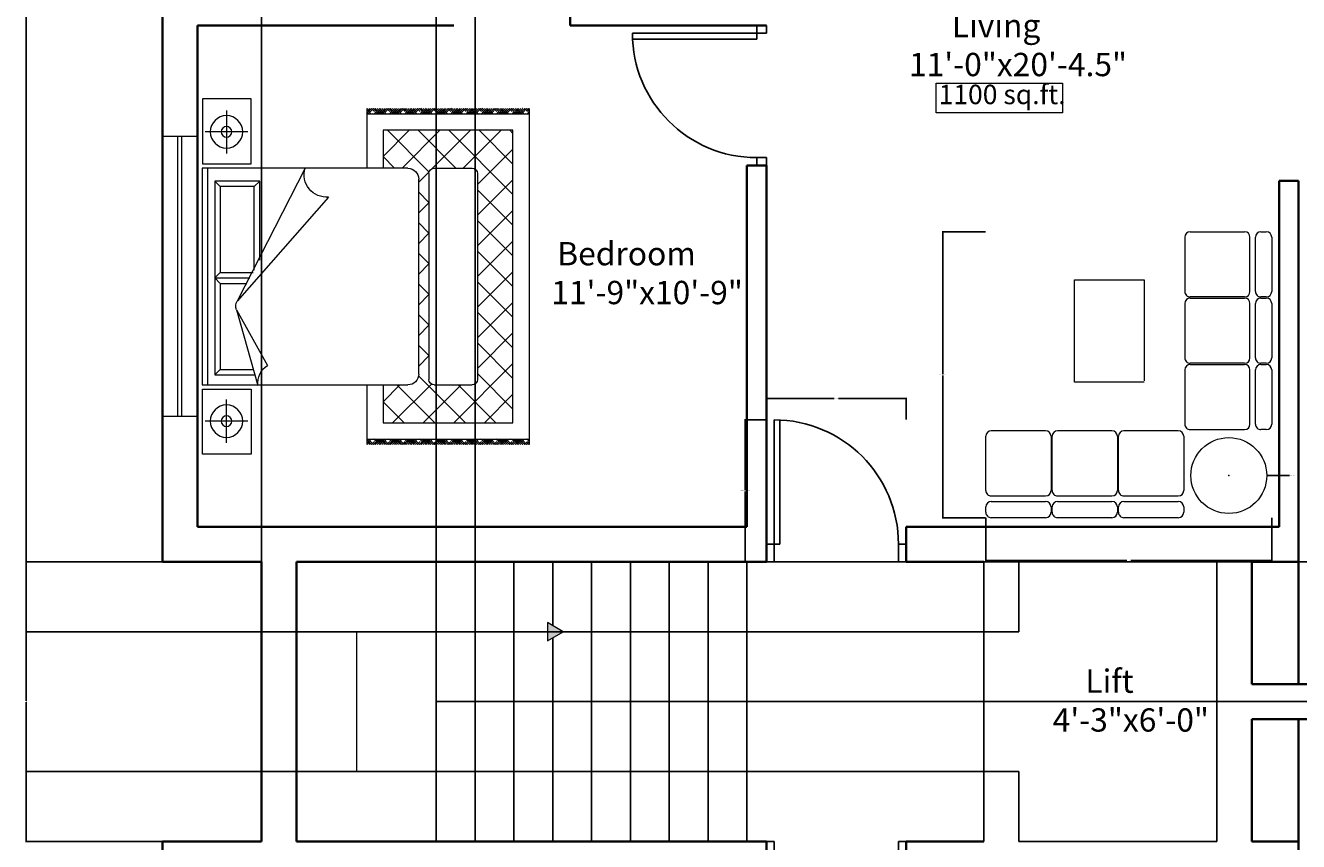
# Model space of a CAD drawing. Units: inches. Extents: x 3198 to 3702, y 1509 to 2253.
# Tile 4 of 6: x 3198 to 3526, y 1845 to 2055. Entities that reach past the tile are written whole.
import ezdxf

# ---------------------------------------------------------------- set-up
doc = ezdxf.new("R2010")
doc.units = ezdxf.units.IN
for name, color, linetype, lineweight in [('A-ANNO-DIMS', 2, 'Continuous', 18), ('A-ANNO-SYMB', 7, 'Continuous', 18), ('A-AREA-IDEN', 7, 'Continuous', 18), ('A-DOOR', 3, 'Continuous', 25), ('A-FLOR-EVTR', 7, 'Continuous', 25), ('A-FLOR-STRS', 7, 'Continuous', 25), ('A-FURN', 8, 'Continuous', 13), ('A-GLAZ', 4, 'Continuous', 18), ('A-WALL', 7, 'Continuous', 35)]:
    doc.layers.add(name, color=color, linetype=linetype, lineweight=lineweight)
doc.styles.get("Standard").update_dxf_attribs({"font": 'arial.ttf'})
doc.dimstyles.get("Standard").update_dxf_attribs({"dimtxt": 0.18, "dimasz": 0.18, "dimexe": 0.18, "dimexo": 0.0625, "dimgap": 0.09, "dimtad": 0, "dimtih": 1, "dimtoh": 1, "dimdec": 4, "dimzin": 0, "dimdsep": 46, "dimtxsty": 'Standard', "dimcen": 0.09, "dimadec": 0, "dimazin": 0, "dimtfac": 1, "dimtdec": 4, "dimtofl": 0, "dimtmove": 0, "dimatfit": 3, "dimfxl": 1, "dimtolj": 1, "dimtzin": 0, "dimarcsym": 0})

# ---------------------------------------------------------------- blocks, each defined once
blk = doc.blocks.new('A$C753D6792')
at = {"linetype": 'ByBlock'}
for p, q in [((0, 2530), (0, 2580)), ((50, 2630), (550, 2630)), ((600, 2580), (600, 2530)), ((610, 2530), (610, 2580)), ((660, 2630), (1160, 2630)), ((1210, 2580), (1210, 2530)), ((1220, 2530), (1220, 2580)), ((1270, 2630), (1770, 2630)), ((1820, 2580), (1820, 2530)), ((550, 2480), (50, 2480)), ((1160, 2480), (660, 2480)), ((1770, 2480), (1270, 2480)), ((0, 1880), (0, 2380)), ((550, 2430), (50, 2430)), ((600, 2380), (600, 1880)), ((610, 1880), (610, 2380)), ((1160, 2430), (660, 2430)), ((1210, 2380), (1210, 1880)), ((1220, 1880), (1220, 2380)), ((1770, 2430), (1270, 2430)), ((1820, 1880), (1820, 2380)), ((50, 1830), (427, 1830)), ((387, 1830), (550, 1830)), ((660, 1830), (1037, 1830)), ((997, 1830), (1160, 1830)), ((1270, 1830), (1647, 1830)), ((1607, 1830), (1770, 1830)), ((1830, 1770), (1830, 1393)), ((1880, 1820), (2380, 1820)), ((2430, 1270), (2430, 1770)), ((2480, 1270), (2480, 1770)), ((2530, 1820), (2580, 1820)), ((2630, 1770), (2630, 1270)), ((442, 815), (442, 1455)), ((442, 1455), (1372, 1455)), ((1382, 1455), (1382, 815)), ((1830, 1433), (1830, 1270)), ((2380, 1220), (1880, 1220)), ((1880, 1210), (2380, 1210)), ((2580, 1220), (2530, 1220)), ((2530, 1210), (2580, 1210)), ((1830, 1160), (1830, 783)), ((2430, 660), (2430, 1160)), ((2480, 660), (2480, 1160)), ((2630, 1160), (2630, 660)), ((1830, 823), (1830, 660)), ((1382, 815), (442, 815)), ((2380, 610), (1880, 610)), ((1880, 600), (2380, 600)), ((2580, 610), (2530, 610)), ((2530, 600), (2580, 600)), ((1830, 550), (1830, 173)), ((2430, 50), (2430, 550)), ((2480, 50), (2480, 550)), ((2630, 550), (2630, 50)), ((1830, 213), (1830, 50)), ((2380, 0), (1880, 0)), ((2580, 0), (2530, 0))]:
    blk.add_line(p, q, dxfattribs=at)
blk.add_circle((2242, 2235), 349, dxfattribs=at)
for centre, start, end in [((50, 2580), 90, 180), ((550, 2580), 0, 90), ((550, 2580), 0, 90), ((660, 2580), 90, 180), ((1160, 2580), 0, 90), ((1160, 2580), 0, 90), ((1270, 2580), 90, 180), ((1770, 2580), 0, 90), ((1770, 2580), 0, 90), ((50, 2530), 180, 270), ((550, 2530), 270, 0), ((550, 2530), 270, 0), ((660, 2530), 180, 270), ((1160, 2530), 270, 0), ((1160, 2530), 270, 0), ((1270, 2530), 180, 270), ((1770, 2530), 270, 0), ((1770, 2530), 270, 0), ((50, 2380), 90, 180), ((550, 2380), 0, 90), ((550, 2380), 0, 90), ((660, 2380), 90, 180), ((1160, 2380), 0, 90), ((1160, 2380), 0, 90), ((1270, 2380), 90, 180), ((1770, 2380), 0, 90), ((1770, 2380), 0, 90), ((50, 1880), 180, 270), ((550, 1880), 270, 0), ((660, 1880), 180, 270), ((1160, 1880), 270, 0), ((1270, 1880), 180, 270), ((1770, 1880), 270, 0), ((1880, 1770), 90, 180), ((2380, 1770), 0, 90), ((2530, 1770), 90, 180), ((2580, 1770), 0, 90), ((1880, 1270), 180, 270), ((1880, 1160), 90, 180), ((2380, 1270), 270, 0), ((2380, 1270), 270, 0), ((2380, 1160), 0, 90), ((2530, 1270), 180, 270), ((2530, 1270), 180, 270), ((2530, 1160), 90, 180), ((2580, 1270), 270, 0), ((2580, 1270), 270, 0), ((2580, 1160), 0, 90), ((1880, 660), 180, 270), ((1880, 550), 90, 180), ((2380, 660), 270, 0), ((2380, 660), 270, 0), ((2380, 550), 0, 90), ((2530, 660), 180, 270), ((2530, 660), 180, 270), ((2530, 550), 90, 180), ((2580, 660), 270, 0), ((2580, 660), 270, 0), ((2580, 550), 0, 90), ((1880, 50), 180, 270), ((2380, 50), 270, 0), ((2380, 50), 270, 0), ((2530, 50), 180, 270), ((2530, 50), 180, 270), ((2580, 50), 270, 0), ((2580, 50), 270, 0)]:
    blk.add_arc(centre, 50, start, end, dxfattribs=at)
blk = doc.blocks.new('A$C4CB008C5')
for p, q in [((0, 3.019), (0.6, 3.019)), ((0, 2.569), (0, 3.019)), ((0.304, 2.6), (0.304, 2.992)), ((0.6, 3.019), (0.6, 2.569)), ((0.64, 1.121), (0.64, 3.021)), ((0.64, 3.021), (2.64, 3.021)), ((0.64, 2.971), (2.64, 2.971)), ((2.64, 3.021), (2.64, 1.121)), ((3.279, 3.019), (2.679, 3.019)), ((2.679, 3.019), (2.679, 2.569)), ((2.975, 2.6), (2.975, 2.992)), ((3.279, 2.569), (3.279, 3.019)), ((0.759, 2.905), (2.547, 2.905)), ((0.759, 2.489), (0.759, 2.905)), ((0.759, 2.905), (0.809, 2.855)), ((0.809, 2.855), (1.603, 2.855)), ((0.809, 2.539), (0.809, 2.855)), ((1.603, 2.855), (1.653, 2.905)), ((1.603, 2.855), (1.603, 2.551)), ((1.653, 2.905), (1.653, 2.579)), ((1.653, 2.905), (1.703, 2.855)), ((1.703, 2.855), (1.703, 2.607)), ((1.703, 2.855), (2.497, 2.855)), ((2.497, 2.855), (2.547, 2.905)), ((2.497, 2.855), (2.497, 2.556)), ((2.547, 2.905), (2.547, 2.54)), ((0.106, 2.796), (0.503, 2.796)), ((1.946, 2.705), (2.646, 2.507)), ((1.946, 2.705), (2.46, 2.418)), ((3.174, 2.796), (2.776, 2.796)), ((0.64, 2.071), (1.866, 2.698)), ((0.906, 1.854), (1.866, 2.698)), ((0.6, 2.569), (0, 2.569)), ((0.809, 2.539), (0.759, 2.489)), ((1.49, 2.489), (0.759, 2.489)), ((1.58, 2.539), (0.809, 2.539)), ((2.679, 2.569), (3.279, 2.569)), ((0.907, 1.867), (0.919, 1.867)), ((0.09, 1.5), (0.64, 1.5)), ((0.09, 1.491), (0.099, 1.5)), ((0.09, 1.473), (0.116, 1.5)), ((0.09, 1.456), (0.134, 1.5)), ((0.09, 1.474), (0.09, 1.475)), ((0.09, 1.438), (0.126, 1.474)), ((0.117, 1.43), (0.09, 1.457)), ((0.14, 1.389), (0.09, 1.439)), ((0.09, 1.42), (0.099, 1.43)), ((0.14, 1.372), (0.09, 1.422)), ((0.09, 1.368), (0.14, 1.417)), ((0.14, 1.46), (0.108, 1.492)), ((0.117, 1.412), (0.14, 1.435)), ((0.14, 1.478), (0.118, 1.5)), ((0.14, 1.496), (0.135, 1.5)), ((0.14, 1.442), (0.135, 1.448)), ((0.14, 0), (0.14, 1.5)), ((2.64, 1.5), (3.19, 1.5)), ((3.14, 1.496), (3.144, 1.5)), ((3.14, 1.478), (3.162, 1.5)), ((3.14, 1.5), (3.14, 0)), ((3.14, 1.46), (3.171, 1.492)), ((3.14, 1.442), (3.145, 1.448)), ((3.14, 1.389), (3.19, 1.439)), ((3.162, 1.412), (3.14, 1.435)), ((3.14, 1.372), (3.19, 1.422)), ((3.189, 1.368), (3.14, 1.417)), ((3.19, 1.456), (3.145, 1.5)), ((3.19, 1.438), (3.154, 1.474)), ((3.162, 1.43), (3.19, 1.457)), ((3.19, 1.473), (3.163, 1.5)), ((3.19, 1.42), (3.18, 1.43)), ((3.19, 1.491), (3.181, 1.5)), ((3.189, 1.474), (3.19, 1.475)), ((0.14, 1.354), (0.09, 1.404)), ((0.09, 1.35), (0.14, 1.4)), ((0.14, 1.336), (0.09, 1.386)), ((0.09, 1.332), (0.14, 1.382)), ((0.09, 1.314), (0.14, 1.364)), ((0.09, 1.297), (0.126, 1.333)), ((0.09, 1.333), (0.09, 1.333)), ((0.117, 1.288), (0.09, 1.316)), ((0.14, 1.248), (0.09, 1.298)), ((0.14, 1.319), (0.108, 1.35)), ((0.117, 1.271), (0.14, 1.294)), ((0.14, 1.301), (0.135, 1.306)), ((0.29, 1.108), (0.532, 1.35)), ((0.29, 0.15), (0.29, 1.35)), ((0.29, 1.35), (0.64, 1.35)), ((0.674, 0.926), (0.29, 1.31)), ((0.64, 1.243), (0.533, 1.35)), ((2.64, 1.195), (2.795, 1.35)), ((2.64, 1.35), (2.99, 1.35)), ((2.99, 1.156), (2.795, 1.35)), ((2.99, 1.35), (2.99, 0.15)), ((3.14, 1.354), (3.19, 1.404)), ((3.19, 1.35), (3.14, 1.4)), ((3.14, 1.336), (3.19, 1.386)), ((3.19, 1.332), (3.14, 1.382)), ((3.19, 1.314), (3.14, 1.364)), ((3.14, 1.319), (3.171, 1.35)), ((3.14, 1.301), (3.145, 1.306)), ((3.14, 1.248), (3.19, 1.298)), ((3.162, 1.271), (3.14, 1.294)), ((3.19, 1.297), (3.154, 1.333)), ((3.162, 1.288), (3.19, 1.316)), ((3.189, 1.333), (3.19, 1.333)), ((0.09, 1.279), (0.099, 1.288)), ((0.14, 1.23), (0.09, 1.28)), ((0.09, 1.227), (0.14, 1.276)), ((0.14, 1.213), (0.09, 1.263)), ((0.09, 1.208), (0.14, 1.258)), ((0.14, 1.195), (0.09, 1.245)), ((0.09, 1.19), (0.14, 1.24)), ((0.09, 1.173), (0.14, 1.223)), ((0.09, 1.191), (0.09, 1.192)), ((0.09, 1.155), (0.126, 1.191)), ((0.14, 1.177), (0.108, 1.209)), ((2.632, 0.904), (2.99, 1.262)), ((2.99, 0.873), (2.64, 1.223)), ((3.14, 1.23), (3.19, 1.28)), ((3.189, 1.227), (3.14, 1.276)), ((3.14, 1.213), (3.19, 1.263)), ((3.19, 1.208), (3.14, 1.258)), ((3.14, 1.195), (3.19, 1.245)), ((3.19, 1.19), (3.14, 1.24)), ((3.19, 1.173), (3.14, 1.223)), ((3.14, 1.177), (3.171, 1.209)), ((3.19, 1.155), (3.154, 1.191)), ((3.19, 1.279), (3.18, 1.288)), ((3.189, 1.191), (3.19, 1.192)), ((0.117, 1.147), (0.09, 1.174)), ((0.14, 1.107), (0.09, 1.157)), ((0.09, 1.137), (0.099, 1.147)), ((0.14, 1.089), (0.09, 1.139)), ((0.09, 1.085), (0.14, 1.134)), ((0.14, 1.071), (0.09, 1.121)), ((0.09, 1.067), (0.14, 1.117)), ((0.14, 1.054), (0.09, 1.104)), ((0.09, 1.049), (0.14, 1.099)), ((0.09, 1.031), (0.14, 1.081)), ((0.14, 1.036), (0.108, 1.067)), ((0.117, 1.129), (0.14, 1.152)), ((0.14, 1.16), (0.135, 1.165)), ((0.29, 0.825), (0.64, 1.175)), ((3.14, 1.16), (3.145, 1.165)), ((3.14, 1.107), (3.19, 1.157)), ((3.162, 1.129), (3.14, 1.152)), ((3.14, 1.089), (3.19, 1.139)), ((3.189, 1.085), (3.14, 1.134)), ((3.14, 1.071), (3.19, 1.121)), ((3.19, 1.067), (3.14, 1.117)), ((3.14, 1.054), (3.19, 1.104)), ((3.19, 1.049), (3.14, 1.099)), ((3.19, 1.031), (3.14, 1.081)), ((3.14, 1.036), (3.171, 1.067)), ((3.162, 1.147), (3.19, 1.174)), ((3.19, 1.137), (3.18, 1.147)), ((0.09, 1.05), (0.09, 1.051)), ((0.09, 1.014), (0.126, 1.05)), ((0.117, 1.006), (0.09, 1.033)), ((0.14, 0.965), (0.09, 1.015)), ((0.09, 0.996), (0.099, 1.006)), ((0.14, 0.948), (0.09, 0.998)), ((0.09, 0.944), (0.14, 0.993)), ((0.14, 0.93), (0.09, 0.98)), ((0.09, 0.925), (0.14, 0.975)), ((0.14, 0.912), (0.09, 0.962)), ((0.09, 0.908), (0.14, 0.958)), ((0.117, 0.988), (0.14, 1.011)), ((0.14, 1.018), (0.135, 1.023)), ((0.64, 0.677), (0.29, 1.027)), ((0.673, 0.925), (0.769, 1.021)), ((2.54, 1.021), (0.74, 1.021)), ((0.955, 0.928), (0.861, 1.021)), ((0.959, 0.928), (1.052, 1.021)), ((1.238, 0.928), (1.144, 1.021)), ((1.241, 0.928), (1.335, 1.021)), ((1.52, 0.928), (1.427, 1.021)), ((1.524, 0.928), (1.618, 1.021)), ((1.803, 0.928), (1.71, 1.021)), ((1.807, 0.928), (1.9, 1.021)), ((2.086, 0.928), (1.993, 1.021)), ((2.09, 0.928), (2.183, 1.021)), ((2.369, 0.928), (2.276, 1.021)), ((2.373, 0.928), (2.466, 1.021)), ((2.99, 0.59), (2.557, 1.023)), ((2.64, 0.629), (2.99, 0.979)), ((3.14, 1.018), (3.145, 1.023)), ((3.14, 0.965), (3.19, 1.015)), ((3.162, 0.988), (3.14, 1.011)), ((3.14, 0.948), (3.19, 0.998)), ((3.189, 0.944), (3.14, 0.993)), ((3.14, 0.93), (3.19, 0.98)), ((3.19, 0.925), (3.14, 0.975)), ((3.14, 0.912), (3.19, 0.962)), ((3.19, 0.908), (3.14, 0.958)), ((3.19, 1.014), (3.154, 1.05)), ((3.162, 1.006), (3.19, 1.033)), ((3.19, 0.996), (3.18, 1.006)), ((3.189, 1.05), (3.19, 1.051)), ((0.09, 0.89), (0.14, 0.94)), ((0.09, 0.908), (0.09, 0.909)), ((0.09, 0.872), (0.126, 0.908)), ((0.117, 0.864), (0.09, 0.891)), ((0.14, 0.824), (0.09, 0.874)), ((0.09, 0.855), (0.099, 0.864)), ((0.14, 0.806), (0.09, 0.856)), ((0.09, 0.802), (0.14, 0.852)), ((0.14, 0.788), (0.09, 0.838)), ((0.09, 0.784), (0.14, 0.834)), ((0.14, 0.894), (0.108, 0.926)), ((0.117, 0.847), (0.14, 0.869)), ((0.14, 0.877), (0.135, 0.882)), ((0.29, 0.542), (0.643, 0.895)), ((0.64, 0.878), (0.64, 0.528)), ((0.69, 0.928), (2.59, 0.928)), ((2.64, 0.878), (2.64, 0.528)), ((3.19, 0.89), (3.14, 0.94)), ((3.14, 0.894), (3.171, 0.926)), ((3.14, 0.877), (3.145, 0.882)), ((3.14, 0.824), (3.19, 0.874)), ((3.162, 0.847), (3.14, 0.869)), ((3.14, 0.806), (3.19, 0.856)), ((3.189, 0.802), (3.14, 0.852)), ((3.14, 0.788), (3.19, 0.838)), ((3.19, 0.784), (3.14, 0.834)), ((3.19, 0.872), (3.154, 0.908)), ((3.162, 0.864), (3.19, 0.891)), ((3.19, 0.855), (3.18, 0.864)), ((3.189, 0.908), (3.19, 0.909)), ((0.14, 0.771), (0.09, 0.821)), ((0.09, 0.766), (0.14, 0.816)), ((0.09, 0.749), (0.14, 0.799)), ((0.09, 0.767), (0.09, 0.768)), ((0.09, 0.731), (0.126, 0.767)), ((0.117, 0.723), (0.09, 0.75)), ((0.14, 0.682), (0.09, 0.732)), ((0.09, 0.713), (0.099, 0.723)), ((0.14, 0.665), (0.09, 0.715)), ((0.09, 0.661), (0.14, 0.71)), ((0.14, 0.753), (0.108, 0.785)), ((0.117, 0.705), (0.14, 0.728)), ((0.14, 0.735), (0.135, 0.74)), ((0.884, 0.15), (0.29, 0.744)), ((3.14, 0.771), (3.19, 0.821)), ((3.19, 0.766), (3.14, 0.816)), ((3.19, 0.749), (3.14, 0.799)), ((3.14, 0.753), (3.171, 0.785)), ((3.14, 0.735), (3.145, 0.74)), ((3.14, 0.682), (3.19, 0.732)), ((3.162, 0.705), (3.14, 0.728)), ((3.14, 0.665), (3.19, 0.715)), ((3.189, 0.661), (3.14, 0.71)), ((3.19, 0.731), (3.154, 0.767)), ((3.162, 0.723), (3.19, 0.75)), ((3.19, 0.713), (3.18, 0.723)), ((3.189, 0.767), (3.19, 0.768)), ((0.14, 0.647), (0.09, 0.697)), ((0.09, 0.642), (0.14, 0.692)), ((0.14, 0.629), (0.09, 0.679)), ((0.09, 0.625), (0.14, 0.675)), ((0.09, 0.607), (0.14, 0.657)), ((0.09, 0.589), (0.126, 0.626)), ((0.09, 0.626), (0.09, 0.626)), ((0.117, 0.581), (0.09, 0.609)), ((0.14, 0.541), (0.09, 0.591)), ((0.14, 0.612), (0.108, 0.643)), ((0.14, 0.594), (0.135, 0.599)), ((0.29, 0.259), (0.64, 0.609)), ((2.443, 0.15), (2.99, 0.696)), ((2.99, 0.307), (2.64, 0.657)), ((3.14, 0.647), (3.19, 0.697)), ((3.19, 0.642), (3.14, 0.692)), ((3.14, 0.629), (3.19, 0.679)), ((3.19, 0.625), (3.14, 0.675)), ((3.19, 0.607), (3.14, 0.657)), ((3.14, 0.612), (3.171, 0.643)), ((3.14, 0.594), (3.145, 0.599)), ((3.14, 0.541), (3.19, 0.591)), ((3.19, 0.589), (3.154, 0.626)), ((3.162, 0.581), (3.19, 0.609)), ((3.189, 0.626), (3.19, 0.626)), ((0.09, 0.572), (0.099, 0.581)), ((0.14, 0.523), (0.09, 0.573)), ((0.09, 0.519), (0.14, 0.569)), ((0.14, 0.506), (0.09, 0.556)), ((0.09, 0.501), (0.14, 0.551)), ((0.14, 0.488), (0.09, 0.538)), ((0.09, 0.483), (0.14, 0.533)), ((0.09, 0.466), (0.14, 0.516)), ((0.09, 0.484), (0.09, 0.485)), ((0.09, 0.448), (0.126, 0.484)), ((0.14, 0.47), (0.108, 0.502)), ((0.117, 0.564), (0.14, 0.586)), ((0.463, 0.15), (0.791, 0.478)), ((0.69, 0.478), (2.59, 0.478)), ((0.746, 0.15), (1.074, 0.478)), ((1.167, 0.15), (0.839, 0.478)), ((1.029, 0.15), (1.357, 0.478)), ((1.45, 0.15), (1.122, 0.478)), ((1.312, 0.15), (1.64, 0.478)), ((1.733, 0.15), (1.405, 0.478)), ((1.595, 0.15), (1.923, 0.478)), ((2.016, 0.15), (1.688, 0.478)), ((1.878, 0.15), (2.206, 0.478)), ((2.298, 0.15), (1.97, 0.478)), ((2.16, 0.15), (2.488, 0.478)), ((2.581, 0.15), (2.253, 0.478)), ((2.864, 0.15), (2.536, 0.478)), ((3.162, 0.564), (3.14, 0.586)), ((3.14, 0.523), (3.19, 0.573)), ((3.189, 0.519), (3.14, 0.569)), ((3.14, 0.506), (3.19, 0.556)), ((3.19, 0.501), (3.14, 0.551)), ((3.14, 0.488), (3.19, 0.538)), ((3.19, 0.483), (3.14, 0.533)), ((3.19, 0.466), (3.14, 0.516)), ((3.14, 0.47), (3.171, 0.502)), ((3.19, 0.448), (3.154, 0.484)), ((3.19, 0.572), (3.18, 0.581)), ((3.189, 0.484), (3.19, 0.485)), ((0.117, 0.44), (0.09, 0.467)), ((0.14, 0.399), (0.09, 0.449)), ((0.09, 0.43), (0.099, 0.44)), ((0.14, 0.382), (0.09, 0.432)), ((0.09, 0.378), (0.14, 0.427)), ((0.14, 0.364), (0.09, 0.414)), ((0.09, 0.36), (0.14, 0.41)), ((0.14, 0.346), (0.09, 0.396)), ((0.09, 0.342), (0.14, 0.392)), ((0.09, 0.324), (0.14, 0.374)), ((0.14, 0.329), (0.108, 0.36)), ((0.117, 0.422), (0.14, 0.445)), ((0.14, 0.453), (0.135, 0.458)), ((0.601, 0.15), (0.29, 0.462)), ((2.726, 0.15), (2.99, 0.414)), ((3.14, 0.453), (3.145, 0.458)), ((3.14, 0.399), (3.19, 0.449)), ((3.162, 0.422), (3.14, 0.445)), ((3.14, 0.382), (3.19, 0.432)), ((3.189, 0.378), (3.14, 0.427)), ((3.14, 0.364), (3.19, 0.414)), ((3.19, 0.36), (3.14, 0.41)), ((3.14, 0.346), (3.19, 0.396)), ((3.19, 0.342), (3.14, 0.392)), ((3.19, 0.324), (3.14, 0.374)), ((3.14, 0.329), (3.171, 0.36)), ((3.162, 0.44), (3.19, 0.467)), ((3.19, 0.43), (3.18, 0.44)), ((0.09, 0.307), (0.126, 0.343)), ((0.09, 0.343), (0.09, 0.343)), ((0.117, 0.299), (0.09, 0.326)), ((0.14, 0.258), (0.09, 0.308)), ((0.09, 0.289), (0.099, 0.299)), ((0.14, 0.24), (0.09, 0.29)), ((0.09, 0.237), (0.14, 0.286)), ((0.14, 0.223), (0.09, 0.273)), ((0.09, 0.218), (0.14, 0.268)), ((0.14, 0.205), (0.09, 0.255)), ((0.09, 0.201), (0.14, 0.251)), ((0.117, 0.281), (0.14, 0.304)), ((0.14, 0.311), (0.135, 0.316)), ((3.14, 0.311), (3.145, 0.316)), ((3.14, 0.258), (3.19, 0.308)), ((3.162, 0.281), (3.14, 0.304)), ((3.14, 0.24), (3.19, 0.29)), ((3.189, 0.237), (3.14, 0.286)), ((3.14, 0.223), (3.19, 0.273)), ((3.19, 0.218), (3.14, 0.268)), ((3.14, 0.205), (3.19, 0.255)), ((3.19, 0.201), (3.14, 0.251)), ((3.19, 0.307), (3.154, 0.343)), ((3.162, 0.299), (3.19, 0.326)), ((3.19, 0.289), (3.18, 0.299)), ((3.189, 0.343), (3.19, 0.343)), ((0.09, 0.183), (0.14, 0.233)), ((0.09, 0.201), (0.09, 0.202)), ((0.09, 0.165), (0.126, 0.201)), ((0.117, 0.157), (0.09, 0.184)), ((0.14, 0.117), (0.09, 0.167)), ((0.09, 0.148), (0.099, 0.157)), ((0.14, 0.099), (0.09, 0.149)), ((0.09, 0.095), (0.14, 0.144)), ((0.14, 0.081), (0.09, 0.131)), ((0.09, 0.077), (0.14, 0.127)), ((0.14, 0.187), (0.108, 0.219)), ((0.117, 0.139), (0.14, 0.162)), ((0.14, 0.17), (0.135, 0.175)), ((0.318, 0.15), (0.29, 0.179)), ((2.99, 0.15), (0.29, 0.15)), ((3.19, 0.183), (3.14, 0.233)), ((3.14, 0.187), (3.171, 0.219)), ((3.14, 0.17), (3.145, 0.175)), ((3.14, 0.117), (3.19, 0.167)), ((3.162, 0.139), (3.14, 0.162)), ((3.14, 0.099), (3.19, 0.149)), ((3.189, 0.095), (3.14, 0.144)), ((3.14, 0.081), (3.19, 0.131)), ((3.19, 0.077), (3.14, 0.127)), ((3.19, 0.165), (3.154, 0.201)), ((3.162, 0.157), (3.19, 0.184)), ((3.19, 0.148), (3.18, 0.157)), ((3.189, 0.201), (3.19, 0.202)), ((0.14, 0.064), (0.09, 0.114)), ((0.09, 0.059), (0.14, 0.109)), ((0.09, 0.041), (0.14, 0.091)), ((0.09, 0.06), (0.09, 0.061)), ((0.09, 0.024), (0.126, 0.06)), ((0.117, 0.016), (0.09, 0.043)), ((0.115, 0), (0.09, 0.025)), ((0.09, 0.006), (0.099, 0.016)), ((0.097, 0), (0.09, 0.008)), ((0.14, 0.046), (0.108, 0.078)), ((0.119, 0), (0.14, 0.021)), ((0.14, 0.028), (0.135, 0.033)), ((0.137, 0), (0.14, 0.003)), ((3.14, 0.064), (3.19, 0.114)), ((3.19, 0.059), (3.14, 0.109)), ((3.19, 0.041), (3.14, 0.091)), ((3.14, 0.046), (3.171, 0.078)), ((3.14, 0.028), (3.145, 0.033)), ((3.16, 0), (3.14, 0.021)), ((3.143, 0), (3.14, 0.003)), ((3.19, 0.024), (3.154, 0.06)), ((3.162, 0.016), (3.19, 0.043)), ((3.164, 0), (3.19, 0.025)), ((3.19, 0.006), (3.18, 0.016)), ((3.182, 0), (3.19, 0.008)), ((3.189, 0.06), (3.19, 0.061)), ((0.09, 0), (3.19, 0))]:
    blk.add_line(p, q)
for centre, radius in [((0.304, 2.796), 0.15), ((2.975, 2.796), 0.15), ((0.304, 2.796), 0.05), ((2.975, 2.796), 0.05)]:
    blk.add_circle(centre, radius)
for centre, radius, start, end in [((1.915, 2.61), 0.1, 71.7215, 119.0799), ((2.626, 2.31), 0.198, 84.1725, 146.9889), ((0.7, 1.873), 0.207, 354.6422, 106.9775), ((0.74, 1.121), 0.1, 180, 270), ((2.54, 1.121), 0.1, 270, 0), ((0.69, 0.878), 0.05, 90, 180), ((2.59, 0.878), 0.05, 0, 90), ((0.69, 0.528), 0.05, 180, 270), ((2.59, 0.528), 0.05, 270, 0)]:
    blk.add_arc(centre, radius, start, end)
blk = doc.blocks.new('DOOR-SINGLE-32')
for p, q in [((0, 34), (32, 34)), ((32, 36), (32, 34)), ((32, 34), (34.5, 34)), ((32, 32.5), (32, 34)), ((34.5, 34), (34.5, 36)), ((0.04, 32.5), (32, 32.5)), ((32, 0), (32, 2)), ((32, 2), (34.5, 2)), ((34.5, 2), (34.5, 0))]:
    blk.add_line(p, q)
blk.add_arc((32, 34), 32, 180, 270)
blk = doc.blocks.new('WIN-72-W9')
for p, q in [((0, 0), (0, 9)), ((72, 0), (72, 9)), ((72, 5), (0, 5)), ((72, 4), (0, 4))]:
    blk.add_line(p, q)
blk = doc.blocks.new('DOOR-ENTRY-32')
for p, q in [((2, 36.5), (2, 4.5)), ((3.5, 36.46), (3.5, 4.5)), ((0, 4.5), (2, 4.5)), ((2, 4.5), (2, 0)), ((2, 4.5), (3.5, 4.5)), ((36, 4.5), (34, 4.5)), ((34, 4.5), (34, 0)), ((2, 0), (0, 0)), ((34, 0), (36, 0))]:
    blk.add_line(p, q)
blk.add_arc((2, 4.5), 32, 360, 90)
blk = doc.blocks.new('*D31')
at = {"layer": 'A-ANNO-DIMS', "color": 0, "lineweight": -2, "transparency": 16777216}
for p, q in [((3444.98, 2001.81), (3433.83, 2001.81)), ((3434.01, 2001.63), (3434.01, 1965.19)), ((3434.01, 1928.39), (3434.01, 1964.83)), ((3444.98, 1928.21), (3433.83, 1928.21))]:
    blk.add_line(p, q, dxfattribs=at)
at = {"layer": 'A-ANNO-DIMS', "color": 0, "transparency": 16777216}
for points in [[(3433.98, 2001.63), (3434.04, 2001.63), (3434.01, 2001.81)], [(3433.98, 1928.39), (3434.04, 1928.39), (3434.01, 1928.21)]]:
    blk.add_solid(points, dxfattribs=at)
at = {"layer": 'Defpoints', "color": 0, "transparency": 16777216}
for p in [(3445.05, 2001.81), (3434.01, 1928.21), (3445.05, 1928.21)]:
    blk.add_point(p, dxfattribs=at)
at = {"layer": 'A-ANNO-DIMS', "color": 0, "transparency": 16777216, "insert": (3434.01, 1965.01), "char_height": 0.18, "attachment_point": 5}
blk.add_mtext('\\A1;SEATING 74 TYP.', dxfattribs=at)
blk = doc.blocks.new('*D32')
at = {"layer": 'A-ANNO-DIMS', "color": 0, "lineweight": -2, "transparency": 16777216}
for p, q in [((3445.05, 1928.15), (3445.05, 1916.99)), ((3518.65, 1928.15), (3518.65, 1916.99)), ((3445.23, 1917.17), (3481.32, 1917.17)), ((3518.47, 1917.17), (3482.37, 1917.17))]:
    blk.add_line(p, q, dxfattribs=at)
at = {"layer": 'A-ANNO-DIMS', "color": 0, "transparency": 16777216}
for points in [[(3445.23, 1917.2), (3445.23, 1917.14), (3445.05, 1917.17)], [(3518.47, 1917.2), (3518.47, 1917.14), (3518.65, 1917.17)]]:
    blk.add_solid(points, dxfattribs=at)
at = {"layer": 'Defpoints', "color": 0, "transparency": 16777216}
for p in [(3445.05, 1928.21), (3518.65, 1928.21), (3518.65, 1917.17)]:
    blk.add_point(p, dxfattribs=at)
at = {"layer": 'A-ANNO-DIMS', "color": 0, "transparency": 16777216, "insert": (3481.85, 1917.17), "char_height": 0.18, "attachment_point": 5}
blk.add_mtext('\\A1;74 TYP.', dxfattribs=at)
blk = doc.blocks.new('*D39')
at = {"layer": 'A-ANNO-DIMS', "color": 0, "lineweight": -2, "transparency": 16777216}
for p, q in [((3388.48, 1953.39), (3382.89, 1953.39)), ((3383.07, 1953.21), (3383.07, 1935.32)), ((3383.07, 1917.07), (3383.07, 1934.95)), ((3388.48, 1916.89), (3382.89, 1916.89))]:
    blk.add_line(p, q, dxfattribs=at)
at = {"layer": 'A-ANNO-DIMS', "color": 0, "transparency": 16777216}
for points in [[(3383.04, 1953.21), (3383.1, 1953.21), (3383.07, 1953.39)], [(3383.04, 1917.07), (3383.1, 1917.07), (3383.07, 1916.89)]]:
    blk.add_solid(points, dxfattribs=at)
at = {"layer": 'Defpoints', "color": 0, "transparency": 16777216}
for p in [(3383.07, 1953.39), (3388.55, 1953.39), (3388.55, 1916.89)]:
    blk.add_point(p, dxfattribs=at)
at = {"layer": 'A-ANNO-DIMS', "color": 0, "transparency": 16777216, "insert": (3383.07, 1935.14), "char_height": 0.18, "attachment_point": 5}
blk.add_mtext('\\A1;ENTRY DOOR 37 TYP.', dxfattribs=at)
blk = doc.blocks.new('*D40')
at = {"layer": 'A-ANNO-DIMS', "color": 0, "lineweight": -2, "transparency": 16777216}
for p, q in [((3388.55, 1953.45), (3388.55, 1959.04)), ((3388.73, 1958.86), (3406.02, 1958.86)), ((3424.37, 1958.86), (3407.08, 1958.86)), ((3424.55, 1953.45), (3424.55, 1959.04))]:
    blk.add_line(p, q, dxfattribs=at)
at = {"layer": 'A-ANNO-DIMS', "color": 0, "transparency": 16777216}
for points in [[(3388.73, 1958.89), (3388.73, 1958.83), (3388.55, 1958.86)], [(3424.37, 1958.89), (3424.37, 1958.83), (3424.55, 1958.86)]]:
    blk.add_solid(points, dxfattribs=at)
at = {"layer": 'Defpoints', "color": 0, "transparency": 16777216}
for p in [(3424.55, 1958.86), (3388.55, 1953.39), (3424.55, 1953.39)]:
    blk.add_point(p, dxfattribs=at)
at = {"layer": 'A-ANNO-DIMS', "color": 0, "transparency": 16777216, "insert": (3406.55, 1958.86), "char_height": 0.18, "attachment_point": 5}
blk.add_mtext('\\A1;36 TYP.', dxfattribs=at)
blk = doc.blocks.new('*D48')
at = {"layer": 'A-ANNO-DIMS', "color": 0, "lineweight": -2, "transparency": 16777216}
for p, q in [((3232.98, 2205.89), (3197.82, 2205.89)), ((3198, 2205.71), (3198, 2061.57)), ((3198, 1917.07), (3198, 2061.21)), ((3232.98, 1916.89), (3197.82, 1916.89))]:
    blk.add_line(p, q, dxfattribs=at)
at = {"layer": 'A-ANNO-DIMS', "color": 0, "transparency": 16777216}
for points in [[(3197.97, 2205.71), (3198.03, 2205.71), (3198, 2205.89)], [(3197.97, 1917.07), (3198.03, 1917.07), (3198, 1916.89)]]:
    blk.add_solid(points, dxfattribs=at)
at = {"layer": 'Defpoints', "color": 0, "transparency": 16777216}
for p in [(3233.05, 2205.89), (3198, 1916.89), (3233.05, 1916.89)]:
    blk.add_point(p, dxfattribs=at)
at = {"layer": 'A-ANNO-DIMS', "color": 0, "transparency": 16777216, "insert": (3198, 2061.39), "char_height": 0.18, "attachment_point": 5}
blk.add_mtext('\\A1;289', dxfattribs=at)
blk = doc.blocks.new('*D49')
at = {"layer": 'A-ANNO-DIMS', "color": 0, "lineweight": -2, "transparency": 16777216}
for p, q in [((3232.98, 1916.89), (3197.82, 1916.89)), ((3198, 1916.71), (3198, 1881.07)), ((3198, 1845.07), (3198, 1880.71)), ((3232.98, 1844.89), (3197.82, 1844.89))]:
    blk.add_line(p, q, dxfattribs=at)
at = {"layer": 'A-ANNO-DIMS', "color": 0, "transparency": 16777216}
for points in [[(3197.97, 1916.71), (3198.03, 1916.71), (3198, 1916.89)], [(3197.97, 1845.07), (3198.03, 1845.07), (3198, 1844.89)]]:
    blk.add_solid(points, dxfattribs=at)
at = {"layer": 'Defpoints', "color": 0, "transparency": 16777216}
for p in [(3233.05, 1916.89), (3198, 1844.89), (3233.05, 1844.89)]:
    blk.add_point(p, dxfattribs=at)
at = {"layer": 'A-ANNO-DIMS', "color": 0, "transparency": 16777216, "insert": (3198, 1880.89), "char_height": 0.18, "attachment_point": 5}
blk.add_mtext('\\A1;72', dxfattribs=at)
blk = doc.blocks.new('*D53')
at = {"layer": 'A-ANNO-DIMS', "color": 0, "lineweight": -2, "transparency": 16777216}
for p, q in [((3233.05, 1916.95), (3233.05, 2252.62)), ((3233.23, 2252.44), (3245.47, 2252.44)), ((3258.37, 2252.44), (3246.12, 2252.44)), ((3258.55, 1916.95), (3258.55, 2252.62))]:
    blk.add_line(p, q, dxfattribs=at)
at = {"layer": 'A-ANNO-DIMS', "color": 0, "transparency": 16777216}
for points in [[(3233.23, 2252.47), (3233.23, 2252.41), (3233.05, 2252.44)], [(3258.37, 2252.47), (3258.37, 2252.41), (3258.55, 2252.44)]]:
    blk.add_solid(points, dxfattribs=at)
at = {"layer": 'Defpoints', "color": 0, "transparency": 16777216}
for p in [(3258.55, 2252.44), (3233.05, 1916.89), (3258.55, 1916.89)]:
    blk.add_point(p, dxfattribs=at)
at = {"layer": 'A-ANNO-DIMS', "color": 0, "transparency": 16777216, "insert": (3245.8, 2252.44), "char_height": 0.18, "attachment_point": 5}
blk.add_mtext('\\A1;25.5', dxfattribs=at)
blk = doc.blocks.new('*D54')
at = {"layer": 'A-ANNO-DIMS', "color": 0, "lineweight": -2, "transparency": 16777216}
for p, q in [((3303.55, 1916.95), (3303.55, 2252.62)), ((3303.73, 2252.44), (3308.34, 2252.44)), ((3313.37, 2252.44), (3308.76, 2252.44)), ((3313.55, 1916.95), (3313.55, 2252.62))]:
    blk.add_line(p, q, dxfattribs=at)
at = {"layer": 'A-ANNO-DIMS', "color": 0, "transparency": 16777216}
for points in [[(3303.73, 2252.47), (3303.73, 2252.41), (3303.55, 2252.44)], [(3313.37, 2252.47), (3313.37, 2252.41), (3313.55, 2252.44)]]:
    blk.add_solid(points, dxfattribs=at)
at = {"layer": 'Defpoints', "color": 0, "transparency": 16777216}
for p in [(3313.55, 2252.44), (3303.55, 1916.89), (3313.55, 1916.89)]:
    blk.add_point(p, dxfattribs=at)
at = {"layer": 'A-ANNO-DIMS', "color": 0, "transparency": 16777216, "insert": (3308.55, 2252.44), "char_height": 0.18, "attachment_point": 5}
blk.add_mtext('\\A1;10', dxfattribs=at)
blk = doc.blocks.new('*D55')
at = {"layer": 'A-ANNO-DIMS', "color": 0, "lineweight": -2, "transparency": 16777216}
for p, q in [((3383.61, 1916.89), (3701.78, 1916.89)), ((3701.6, 1916.71), (3701.6, 1899.07)), ((3701.6, 1881.07), (3701.6, 1898.71)), ((3383.61, 1880.89), (3701.78, 1880.89))]:
    blk.add_line(p, q, dxfattribs=at)
at = {"layer": 'A-ANNO-DIMS', "color": 0, "transparency": 16777216}
for points in [[(3701.57, 1916.71), (3701.63, 1916.71), (3701.6, 1916.89)], [(3701.57, 1881.07), (3701.63, 1881.07), (3701.6, 1880.89)]]:
    blk.add_solid(points, dxfattribs=at)
at = {"layer": 'Defpoints', "color": 0, "transparency": 16777216}
for p in [(3383.55, 1916.89), (3701.6, 1916.89), (3383.55, 1880.89)]:
    blk.add_point(p, dxfattribs=at)
at = {"layer": 'A-ANNO-DIMS', "color": 0, "transparency": 16777216, "insert": (3701.6, 1898.89), "char_height": 0.18, "attachment_point": 5}
blk.add_mtext('\\A1;36', dxfattribs=at)
blk = doc.blocks.new('*D56')
at = {"layer": 'A-ANNO-DIMS', "color": 0, "lineweight": -2, "transparency": 16777216}
for p, q in [((3444.48, 1898.89), (3197.82, 1898.89)), ((3198, 1898.71), (3198, 1881.07)), ((3198, 1863.07), (3198, 1880.71)), ((3444.48, 1862.89), (3197.82, 1862.89))]:
    blk.add_line(p, q, dxfattribs=at)
at = {"layer": 'A-ANNO-DIMS', "color": 0, "transparency": 16777216}
for points in [[(3197.97, 1898.71), (3198.03, 1898.71), (3198, 1898.89)], [(3197.97, 1863.07), (3198.03, 1863.07), (3198, 1862.89)]]:
    blk.add_solid(points, dxfattribs=at)
at = {"layer": 'Defpoints', "color": 0, "transparency": 16777216}
for p in [(3198, 1898.89), (3444.55, 1898.89), (3444.55, 1862.89)]:
    blk.add_point(p, dxfattribs=at)
at = {"layer": 'A-ANNO-DIMS', "color": 0, "transparency": 16777216, "insert": (3198, 1880.89), "char_height": 0.18, "attachment_point": 5}
blk.add_mtext('\\A1;36', dxfattribs=at)
blk = doc.blocks.new('*D66')
at = {"layer": 'A-ANNO-DIMS', "color": 0, "lineweight": -2, "transparency": 16777216}
for p, q in [((3507.5, 1939.06), (3507.68, 1939.06)), ((3507.59, 1938.97), (3507.59, 1939.15)), ((3523.23, 1939.06), (3517.55, 1939.06))]:
    blk.add_line(p, q, dxfattribs=at)
at = {"layer": 'A-ANNO-DIMS', "color": 0, "transparency": 16777216}
blk.add_solid([(3517.55, 1939.09), (3517.55, 1939.03), (3517.37, 1939.06)], dxfattribs=at)
at = {"layer": 'Defpoints', "color": 0, "transparency": 16777216}
for p in [(3497.82, 1939.06), (3517.37, 1939.06)]:
    blk.add_point(p, dxfattribs=at)
at = {"layer": 'A-ANNO-DIMS', "color": 0, "transparency": 16777216, "insert": (3523.91, 1939.06), "char_height": 0.18, "attachment_point": 5}
blk.add_mtext('\\A1;2X ∅19.55', dxfattribs=at)

msp = doc.modelspace()

# ---------------------------------------------------------------- hatches: boundary and pattern name
at = {"layer": 'A-ANNO-SYMB'}
h = msp.add_hatch(color=256, dxfattribs=at)
h.dxf.hatch_style = 1
h.paths.add_polyline_path([(3332.1962, 1901.2285), (3332.1962, 1896.5475), (3336.25, 1898.888)])

# ---------------------------------------------------------------- linework, layer by layer
for p, q in [((3283.0266, 1898.888), (3332.1962, 1898.888)), ((3283.0266, 1898.888), (3283.0266, 1862.888)), ((3283.0266, 1862.888), (3383.5475, 1862.888))]:
    msp.add_line(p, q, dxfattribs=at)
msp.add_lwpolyline([(3336.25, 1898.888), (3332.1962, 1901.2285), (3332.1962, 1896.5475)], close=True, dxfattribs=at)
at = {"layer": 'A-AREA-IDEN'}
msp.add_lwpolyline([(3432.2919, 2040.074), (3464.7788, 2040.074), (3464.7788, 2032.3662), (3432.2919, 2032.3662)], close=True, dxfattribs=at)
at = {"layer": 'A-FLOR-EVTR'}
for p, q in [((3444.5475, 1916.888), (3444.5475, 1844.888)), ((3453.5475, 1916.888), (3453.5475, 1898.888)), ((3453.5475, 1916.888), (3504.5475, 1916.888)), ((3504.5475, 1916.888), (3504.5475, 1844.888)), ((3453.5475, 1898.888), (3444.5475, 1898.888)), ((3453.5475, 1862.888), (3444.5475, 1862.888)), ((3453.5475, 1862.888), (3453.5475, 1844.888)), ((3453.5475, 1844.888), (3504.5475, 1844.888))]:
    msp.add_line(p, q, dxfattribs=at)
at = {"layer": 'A-FLOR-STRS'}
for p, q in [((3303.5475, 1916.888), (3303.5475, 1844.888)), ((3313.5475, 1916.888), (3313.5475, 1844.888)), ((3323.5475, 1916.888), (3323.5475, 1844.888)), ((3333.5475, 1916.888), (3333.5475, 1900.4483)), ((3343.5475, 1916.888), (3343.5475, 1844.888)), ((3353.5475, 1916.888), (3353.5475, 1844.888)), ((3363.5475, 1916.888), (3363.5475, 1844.888)), ((3373.5475, 1916.888), (3373.5475, 1844.888)), ((3383.5475, 1916.888), (3383.5475, 1844.888)), ((3333.5475, 1897.3277), (3333.5475, 1844.888)), ((3303.5475, 1880.888), (3383.5475, 1880.888))]:
    msp.add_line(p, q, dxfattribs=at)
at = {"layer": 'A-WALL'}
for p, q in [((3233.0475, 2205.888), (3233.0475, 1916.888)), ((3338.0475, 2107.888), (3338.0475, 2054.888)), ((3242.0475, 2054.888), (3308.0475, 2054.888)), ((3242.0475, 2054.888), (3242.0475, 1925.888)), ((3338.0475, 2054.888), (3388.5475, 2054.888)), ((3383.5475, 2018.888), (3388.5475, 2018.888)), ((3383.5475, 2018.888), (3383.5475, 1925.888)), ((3388.5475, 2018.888), (3388.5475, 1916.888)), ((3520.5475, 2014.888), (3525.5475, 2014.888)), ((3520.5475, 2014.888), (3520.5475, 1925.888)), ((3525.5475, 2014.888), (3525.5475, 1885.388)), ((3242.0475, 1925.888), (3383.5475, 1925.888)), ((3424.5475, 1925.888), (3520.5475, 1925.888)), ((3424.5475, 1925.888), (3424.5475, 1916.888)), ((3233.0475, 1916.888), (3258.5475, 1916.888)), ((3258.5475, 1916.888), (3258.5475, 1844.888)), ((3267.5475, 1916.888), (3267.5475, 1844.888)), ((3267.5475, 1916.888), (3388.5475, 1916.888)), ((3424.5475, 1916.888), (3444.5475, 1916.888)), ((3513.5475, 1916.888), (3513.5475, 1885.388)), ((3513.5475, 1916.888), (3525.5475, 1916.888)), ((3513.5475, 1885.388), (3657.5475, 1885.388)), ((3513.5475, 1876.388), (3657.5475, 1876.388)), ((3513.5475, 1876.388), (3513.5475, 1844.888)), ((3525.5475, 1876.388), (3525.5475, 1742.388)), ((3233.0475, 1844.888), (3258.5475, 1844.888)), ((3233.0475, 1844.888), (3233.0475, 1555.888)), ((3267.5475, 1844.888), (3388.5475, 1844.888)), ((3388.5475, 1844.888), (3388.5475, 1787.888)), ((3424.5475, 1844.888), (3424.5475, 1835.888)), ((3424.5475, 1844.888), (3444.5475, 1844.888)), ((3513.5475, 1844.888), (3525.5475, 1844.888))]:
    msp.add_line(p, q, dxfattribs=at)

# ---------------------------------------------------------------- block references
at = {"layer": 'A-DOOR'}
for name, p in [('DOOR-SINGLE-32', (3354.047, 2018.888)), ('DOOR-ENTRY-32', (3388.547, 1916.888))]:
    msp.add_blockref(name, p, dxfattribs=at)
at = {"layer": 'A-DOOR', "extrusion": (0, 0, -1), "zscale": -1, "rotation": 180}
msp.add_blockref('DOOR-ENTRY-32', (-3388.547, 1844.888), dxfattribs=at)
at = {"layer": 'A-FURN'}
for name, p, xscale, yscale, zscale, rotation in [('A$C4CB008C5', (3327.4909, 2035.9921), -27.87562936897135, 27.87562936897135, 27.87562936897135, 90), ('A$C753D6792', (3445.047, 2001.8089), 0.0279847415898772, 0.0279847415898772, 0.0279847415898772, 270)]:
    msp.add_blockref(name, p, dxfattribs=dict(at, xscale=xscale, yscale=yscale, zscale=zscale, rotation=rotation))
at = {"layer": 'A-GLAZ', "rotation": 269.9999999999986}
msp.add_blockref('WIN-72-W9', (3233.0475, 2026.3885), dxfattribs=at)

# ---------------------------------------------------------------- texts
at = {"layer": 'A-AREA-IDEN', "attachment_point": 1}
for s, width, insert, char_height in [('{\\H2.4x;      Living\\P11\'-0"x20\'-4.5"}', 72.249028, (3425.2579, 2057.8436), 2.5), ('1100 sq.ft.', 36.112833, (3432.894, 2039.6364), 5), ('  {\\H2.4x;Bedroom\\P11\'-9"x10\'-9"}', 75.551815, (3333.171, 1999.1699), 2.5), ('           {\\H2.4x;Lift\\P4\'-3"x6\'-0"}', 42.293948, (3462.2535, 1889.1636), 2.5)]:
    msp.add_mtext_dynamic_manual_height_columns(s, width=width, gutter_width=12.5, heights=[0], dxfattribs=dict(at, insert=insert, char_height=char_height))

# ---------------------------------------------------------------- dimensions: what is measured, and where the dimension line sits
at = {"layer": 'A-ANNO-DIMS'}
for base, p1, p2, override, picture, middle in [((3258.5475, 2252.438), (3233.0475, 1916.888), (3258.5475, 1916.888), {"dimdec": 1, "dimlfac": 1, "dimrnd": 0, "dimzin": 0, "dimdsep": 46, "dimlunit": 2}, '*D53', (3245.7975, 2252.438)), ((3313.5475, 2252.438), (3303.5475, 1916.888), (3313.5475, 1916.888), {"dimdec": 0, "dimlfac": 1, "dimrnd": 0, "dimzin": 0, "dimdsep": 46, "dimlunit": 2}, '*D54', (3308.5475, 2252.438))]:
    dim = msp.add_linear_dim(base=base, p1=p1, p2=p2, dimstyle='Standard', override=override, dxfattribs=at)
    dim.commit()
    dim.dimension.update_dxf_attribs({"geometry": picture, "text_midpoint": middle})
for base, p1, p2, picture, middle in [((3197.9975, 1916.888), (3233.0475, 2205.888), (3233.0475, 1916.888), '*D48', (3197.9975, 2061.388)), ((3197.9975, 1844.888), (3233.0475, 1916.888), (3233.0475, 1844.888), '*D49', (3197.9975, 1880.888)), ((3701.5975, 1916.888), (3383.5475, 1880.888), (3383.5475, 1916.888), '*D55', (3701.5975, 1898.888)), ((3197.9975, 1898.888), (3444.5475, 1862.888), (3444.5475, 1898.888), '*D56', (3197.9975, 1880.888))]:
    dim = msp.add_linear_dim(base=base, p1=p1, p2=p2, angle=90, dimstyle='Standard', override={"dimdec": 0, "dimlfac": 1, "dimrnd": 0, "dimzin": 0, "dimdsep": 46, "dimlunit": 2}, dxfattribs=at)
    dim.commit()
    dim.dimension.update_dxf_attribs({"geometry": picture, "text_midpoint": middle})
for base, p1, p2, angle, text, picture, middle in [((3434.007, 1928.2091), (3445.047, 2001.809), (3445.047, 1928.2091), 270, 'SEATING <> TYP.', '*D31', (3434.007, 1965.009)), ((3383.0724569853, 1953.3880023156), (3388.5474569852, 1916.8880023156), (3388.5474569852, 1953.3880023156), 90, 'ENTRY DOOR <> TYP.', '*D39', (3383.0724569853, 1935.1380023156))]:
    dim = msp.add_linear_dim(base=base, p1=p1, p2=p2, angle=angle, text=text, dimstyle='Standard', override={"dimdec": 0, "dimlfac": 1, "dimrnd": 0, "dimzin": 0, "dimdsep": 46, "dimlunit": 2}, dxfattribs=at)
    dim.commit()
    dim.dimension.update_dxf_attribs({"geometry": picture, "text_midpoint": middle})
for base, p1, p2, picture, middle in [((3424.5475, 1958.863), (3388.5475, 1953.388), (3424.5475, 1953.388), '*D40', (3406.5475, 1958.863)), ((3518.6469, 1917.1691), (3445.047, 1928.2091), (3518.6469, 1928.2091), '*D32', (3481.8469, 1917.1691))]:
    dim = msp.add_linear_dim(base=base, p1=p1, p2=p2, text='<> TYP.', dimstyle='Standard', override={"dimdec": 0, "dimlfac": 1, "dimrnd": 0, "dimzin": 0, "dimdsep": 46, "dimlunit": 2}, dxfattribs=at)
    dim.commit()
    dim.dimension.update_dxf_attribs({"geometry": picture, "text_midpoint": middle})
dim = msp.add_diameter_dim_2p(p1=(3497.8183, 1939.0576), p2=(3517.3676, 1939.058), text='2X <>', dimstyle='Standard', override={"dimdec": 2, "dimlfac": 1, "dimrnd": 0, "dimzin": 0, "dimdsep": 46, "dimlunit": 2}, dxfattribs=at)
dim.commit()
dim.dimension.update_dxf_attribs({"geometry": '*D66', "text_midpoint": (3523.2323, 1939.0581), "dimtype": 163})

doc.saveas('drawing.dxf')
